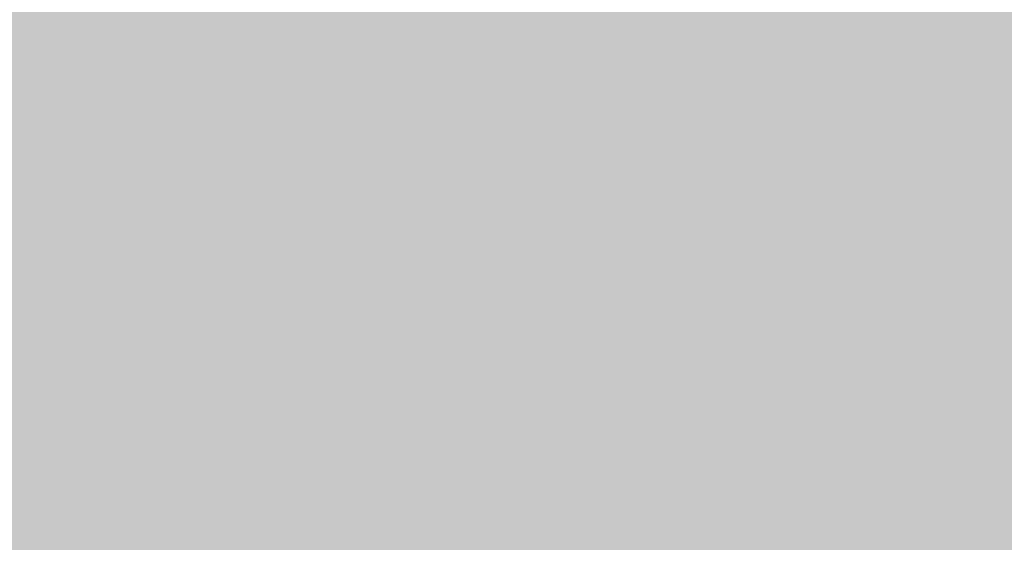
# Model space of a CAD drawing. Units: millimetres. Extents: x -22994 to 29398, y -19990 to 20176.
# Tile 104 of 135: x 223.11 to 237.22, y 87.07 to 94.56. Entities that reach past the tile are written whole.
import ezdxf
from ezdxf import colors
from ezdxf.entities.mleader import LeaderData, LeaderLine
from ezdxf.math import Vec2, Vec3

# ---------------------------------------------------------------- set-up
doc = ezdxf.new("R2010")
doc.units = ezdxf.units.MM
doc.header["$MEASUREMENT"] = 0
doc.layers.add('M-ANNO-TEXT', color=7, linetype='Continuous', lineweight=25)
doc.layers.add('M-DIMS', color=2, linetype='Continuous', lineweight=18)
doc.styles.get("Standard").update_dxf_attribs({"font": 'arial.ttf'})
doc.dimstyles.get("Standard").update_dxf_attribs({"dimtxt": 0.18, "dimasz": 10000, "dimexe": 0.18, "dimexo": 0.0625, "dimgap": 0.09, "dimtad": 0, "dimtih": 1, "dimtoh": 1, "dimdec": 0, "dimzin": 0, "dimdsep": 46, "dimtxsty": 'Standard', "dimcen": 0.09, "dimadec": 0, "dimazin": 0, "dimtfac": 1, "dimtdec": 0, "dimtofl": 0, "dimtmove": 0, "dimatfit": 3, "dimfxl": 1, "dimtolj": 1, "dimtzin": 0, "dimlwd": 30, "dimarcsym": 0})

# ---------------------------------------------------------------- blocks, each defined once
blk = doc.blocks.new('*D2')
at = {"layer": 'Defpoints', "color": 0, "transparency": 16777216}
for p in [(6.677, 10.271), (290.852, 10.271), (290.852, -5.079)]:
    blk.add_point(p, dxfattribs=at)
at = {"layer": 'M-DIMS', "color": 0, "lineweight": -2, "transparency": 16777216}
for p, q in [((6.677, 10.209), (6.677, -5.259)), ((290.852, 10.209), (290.852, -5.259))]:
    blk.add_line(p, q, dxfattribs=at)
at = {"layer": 'M-DIMS', "color": 0, "lineweight": 30, "transparency": 16777216}
for p, q in [((-9993.323, -5.079), (-19993.323, -5.079)), ((10290.852, -5.079), (20290.852, -5.079))]:
    blk.add_line(p, q, dxfattribs=at)
at = {"layer": 'M-DIMS', "color": 0, "transparency": 16777216}
for points in [[(-9993.323, 1661.588), (-9993.323, -1671.745), (6.677, -5.079)], [(10290.852, 1661.588), (10290.852, -1671.745), (290.852, -5.079)]]:
    blk.add_solid(points, dxfattribs=at)
at = {"layer": 'M-DIMS', "color": 0, "transparency": 16777216, "insert": (148.765, -5.079), "char_height": 0.18, "attachment_point": 5}
blk.add_mtext('\\A1;284.2', dxfattribs=at)
blk = doc.blocks.new('*D3')
at = {"layer": 'Defpoints', "color": 0, "transparency": 16777216}
for p in [(110.265, 204.165), (110.265, 176.366), (95.833, 127.967)]:
    blk.add_point(p, dxfattribs=at)
at = {"layer": 'M-DIMS', "color": 0, "lineweight": -2, "transparency": 16777216}
for p, q in [((95.833, 128.03), (95.833, 204.345)), ((110.265, 176.429), (110.265, 204.345))]:
    blk.add_line(p, q, dxfattribs=at)
at = {"layer": 'M-DIMS', "color": 0, "lineweight": 30, "transparency": 16777216}
for p, q in [((-9904.167, 204.165), (-19904.167, 204.165)), ((10110.265, 204.165), (20110.265, 204.165))]:
    blk.add_line(p, q, dxfattribs=at)
at = {"layer": 'M-DIMS', "color": 0, "transparency": 16777216}
for points in [[(-9904.167, 1870.832), (-9904.167, -1462.501), (95.833, 204.165)], [(10110.265, 1870.832), (10110.265, -1462.501), (110.265, 204.165)]]:
    blk.add_solid(points, dxfattribs=at)
at = {"layer": 'M-DIMS', "color": 0, "transparency": 16777216, "insert": (103.049, 204.165), "char_height": 0.18, "attachment_point": 5}
blk.add_mtext('\\A1;14.432', dxfattribs=at)
blk = doc.blocks.new('*D4')
at = {"layer": 'Defpoints', "color": 0, "transparency": 16777216}
for p in [(116.265, 204.165), (110.265, 176.366), (116.265, 176.366)]:
    blk.add_point(p, dxfattribs=at)
at = {"layer": 'M-DIMS', "color": 0, "lineweight": -2, "transparency": 16777216}
for p, q in [((110.265, 176.429), (110.265, 204.345)), ((116.265, 176.429), (116.265, 204.345))]:
    blk.add_line(p, q, dxfattribs=at)
at = {"layer": 'M-DIMS', "color": 0, "lineweight": 30, "transparency": 16777216}
for p, q in [((-9889.735, 204.165), (-19889.735, 204.165)), ((10116.265, 204.165), (20116.265, 204.165))]:
    blk.add_line(p, q, dxfattribs=at)
at = {"layer": 'M-DIMS', "color": 0, "transparency": 16777216}
for points in [[(-9889.735, 1870.832), (-9889.735, -1462.501), (110.265, 204.165)], [(10116.265, 1870.832), (10116.265, -1462.501), (116.265, 204.165)]]:
    blk.add_solid(points, dxfattribs=at)
at = {"layer": 'M-DIMS', "color": 0, "transparency": 16777216, "insert": (113.265, 204.165), "char_height": 0.18, "attachment_point": 5}
blk.add_mtext('\\A1;6', dxfattribs=at)
blk = doc.blocks.new('*D5')
at = {"layer": 'Defpoints', "color": 0, "transparency": 16777216}
for p in [(181.265, 204.165), (116.265, 176.366), (181.265, 176.366)]:
    blk.add_point(p, dxfattribs=at)
at = {"layer": 'M-DIMS', "color": 0, "lineweight": -2, "transparency": 16777216}
for p, q in [((116.265, 176.429), (116.265, 204.345)), ((181.265, 176.429), (181.265, 204.345))]:
    blk.add_line(p, q, dxfattribs=at)
at = {"layer": 'M-DIMS', "color": 0, "lineweight": 30, "transparency": 16777216}
for p, q in [((-9883.735, 204.165), (-19883.735, 204.165)), ((10181.265, 204.165), (20181.265, 204.165))]:
    blk.add_line(p, q, dxfattribs=at)
at = {"layer": 'M-DIMS', "color": 0, "transparency": 16777216}
for points in [[(-9883.735, 1870.832), (-9883.735, -1462.501), (116.265, 204.165)], [(10181.265, 1870.832), (10181.265, -1462.501), (181.265, 204.165)]]:
    blk.add_solid(points, dxfattribs=at)
at = {"layer": 'M-DIMS', "color": 0, "transparency": 16777216, "insert": (148.765, 204.165), "char_height": 0.18, "attachment_point": 5}
blk.add_mtext('\\A1;65', dxfattribs=at)
blk = doc.blocks.new('*D6')
at = {"layer": 'Defpoints', "color": 0, "transparency": 16777216}
for p in [(187.265, 204.165), (181.265, 176.366), (187.265, 176.366)]:
    blk.add_point(p, dxfattribs=at)
at = {"layer": 'M-DIMS', "color": 0, "lineweight": -2, "transparency": 16777216}
for p, q in [((181.265, 176.429), (181.265, 204.345)), ((187.265, 176.429), (187.265, 204.345))]:
    blk.add_line(p, q, dxfattribs=at)
at = {"layer": 'M-DIMS', "color": 0, "lineweight": 30, "transparency": 16777216}
for p, q in [((-9818.735, 204.165), (-19818.735, 204.165)), ((10187.265, 204.165), (20187.265, 204.165))]:
    blk.add_line(p, q, dxfattribs=at)
at = {"layer": 'M-DIMS', "color": 0, "transparency": 16777216}
for points in [[(-9818.735, 1870.832), (-9818.735, -1462.501), (181.265, 204.165)], [(10187.265, 1870.832), (10187.265, -1462.501), (187.265, 204.165)]]:
    blk.add_solid(points, dxfattribs=at)
at = {"layer": 'M-DIMS', "color": 0, "transparency": 16777216, "insert": (184.265, 204.165), "char_height": 0.18, "attachment_point": 5}
blk.add_mtext('\\A1;6', dxfattribs=at)
blk = doc.blocks.new('*D7')
at = {"layer": 'Defpoints', "color": 0, "transparency": 16777216}
for p in [(201.697, 204.165), (187.265, 176.366), (201.697, 127.967)]:
    blk.add_point(p, dxfattribs=at)
at = {"layer": 'M-DIMS', "color": 0, "lineweight": -2, "transparency": 16777216}
for p, q in [((187.265, 176.429), (187.265, 204.345)), ((201.697, 128.03), (201.697, 204.345))]:
    blk.add_line(p, q, dxfattribs=at)
at = {"layer": 'M-DIMS', "color": 0, "lineweight": 30, "transparency": 16777216}
for p, q in [((-9812.735, 204.165), (-19812.735, 204.165)), ((10201.697, 204.165), (20201.697, 204.165))]:
    blk.add_line(p, q, dxfattribs=at)
at = {"layer": 'M-DIMS', "color": 0, "transparency": 16777216}
for points in [[(-9812.735, 1870.832), (-9812.735, -1462.501), (187.265, 204.165)], [(10201.697, 1870.832), (10201.697, -1462.501), (201.697, 204.165)]]:
    blk.add_solid(points, dxfattribs=at)
at = {"layer": 'M-DIMS', "color": 0, "transparency": 16777216, "insert": (194.481, 204.165), "char_height": 0.18, "attachment_point": 5}
blk.add_mtext('\\A1;14.432', dxfattribs=at)
blk = doc.blocks.new('*D8')
at = {"layer": 'Defpoints', "color": 0, "transparency": 16777216}
for p in [(227.648, 204.165), (227.648, 146.73), (201.697, 127.967)]:
    blk.add_point(p, dxfattribs=at)
at = {"layer": 'M-DIMS', "color": 0, "lineweight": -2, "transparency": 16777216}
for p, q in [((201.697, 128.03), (201.697, 204.345)), ((227.648, 146.792), (227.648, 204.345))]:
    blk.add_line(p, q, dxfattribs=at)
at = {"layer": 'M-DIMS', "color": 0, "lineweight": 30, "transparency": 16777216}
for p, q in [((-9798.303, 204.165), (-19798.303, 204.165)), ((10227.648, 204.165), (20227.648, 204.165))]:
    blk.add_line(p, q, dxfattribs=at)
at = {"layer": 'M-DIMS', "color": 0, "transparency": 16777216}
for points in [[(-9798.303, 1870.832), (-9798.303, -1462.501), (201.697, 204.165)], [(10227.648, 1870.832), (10227.648, -1462.501), (227.648, 204.165)]]:
    blk.add_solid(points, dxfattribs=at)
at = {"layer": 'M-DIMS', "color": 0, "transparency": 16777216, "insert": (214.673, 204.165), "char_height": 0.18, "attachment_point": 5}
blk.add_mtext('\\A1;25.95', dxfattribs=at)
blk = doc.blocks.new('*D9')
at = {"layer": 'Defpoints', "color": 0, "transparency": 16777216}
for p in [(187.265, 176.366), (306.202, 176.366), (290.852, 10.271)]:
    blk.add_point(p, dxfattribs=at)
at = {"layer": 'M-DIMS', "color": 0, "lineweight": 30, "transparency": 16777216}
for p, q in [((306.202, 10176.366), (306.202, 20176.366)), ((306.202, -9989.729), (306.202, -19989.729))]:
    blk.add_line(p, q, dxfattribs=at)
at = {"layer": 'M-DIMS', "color": 0, "lineweight": -2, "transparency": 16777216}
for p, q in [((187.327, 176.366), (306.382, 176.366)), ((290.915, 10.271), (306.382, 10.271))]:
    blk.add_line(p, q, dxfattribs=at)
at = {"layer": 'M-DIMS', "color": 0, "transparency": 16777216}
for points in [[(-1360.465, 10176.366), (1972.869, 10176.366), (306.202, 176.366)], [(-1360.465, -9989.729), (1972.869, -9989.729), (306.202, 10.271)]]:
    blk.add_solid(points, dxfattribs=at)
at = {"layer": 'M-DIMS', "color": 0, "transparency": 16777216, "insert": (306.202, 93.319), "char_height": 0.18, "attachment_point": 5}
blk.add_mtext('\\A1;166.1', dxfattribs=at)
blk = doc.blocks.new('*D10')
at = {"layer": 'Defpoints', "color": 0, "transparency": 16777216}
for p in [(125.65, 136.071), (133.346, 136.071), (133.346, -5.079)]:
    blk.add_point(p, dxfattribs=at)
at = {"layer": 'M-DIMS', "color": 0, "lineweight": -2, "transparency": 16777216}
for p, q in [((125.65, 136.009), (125.65, -5.259)), ((133.346, 136.009), (133.346, -5.259))]:
    blk.add_line(p, q, dxfattribs=at)
at = {"layer": 'M-DIMS', "color": 0, "lineweight": 30, "transparency": 16777216}
for p, q in [((-9874.35, -5.079), (-19874.35, -5.079)), ((10133.346, -5.079), (20133.346, -5.079))]:
    blk.add_line(p, q, dxfattribs=at)
at = {"layer": 'M-DIMS', "color": 0, "transparency": 16777216}
for points in [[(-9874.35, 1661.588), (-9874.35, -1671.745), (125.65, -5.079)], [(10133.346, 1661.588), (10133.346, -1671.745), (133.346, -5.079)]]:
    blk.add_solid(points, dxfattribs=at)
at = {"layer": 'M-DIMS', "color": 0, "transparency": 16777216, "insert": (129.498, -5.079), "char_height": 0.18, "attachment_point": 5}
blk.add_mtext('\\A1;7.696', dxfattribs=at)
blk = doc.blocks.new('*D11')
at = {"layer": 'Defpoints', "color": 0, "transparency": 16777216}
for p in [(133.346, 136.071), (135.65, 136.071), (135.65, -5.079)]:
    blk.add_point(p, dxfattribs=at)
at = {"layer": 'M-DIMS', "color": 0, "lineweight": -2, "transparency": 16777216}
for p, q in [((133.346, 136.009), (133.346, -5.259)), ((135.65, 136.009), (135.65, -5.259))]:
    blk.add_line(p, q, dxfattribs=at)
at = {"layer": 'M-DIMS', "color": 0, "lineweight": 30, "transparency": 16777216}
for p, q in [((-9866.654, -5.079), (-19866.654, -5.079)), ((10135.65, -5.079), (20135.65, -5.079))]:
    blk.add_line(p, q, dxfattribs=at)
at = {"layer": 'M-DIMS', "color": 0, "transparency": 16777216}
for points in [[(-9866.654, 1661.588), (-9866.654, -1671.745), (133.346, -5.079)], [(10135.65, 1661.588), (10135.65, -1671.745), (135.65, -5.079)]]:
    blk.add_solid(points, dxfattribs=at)
at = {"layer": 'M-DIMS', "color": 0, "transparency": 16777216, "insert": (134.498, -5.079), "char_height": 0.18, "attachment_point": 5}
blk.add_mtext('\\A1;2.304', dxfattribs=at)
blk = doc.blocks.new('*D12')
at = {"layer": 'Defpoints', "color": 0, "transparency": 16777216}
for p in [(135.65, 136.071), (145.65, 136.071), (145.65, -5.079)]:
    blk.add_point(p, dxfattribs=at)
at = {"layer": 'M-DIMS', "color": 0, "lineweight": -2, "transparency": 16777216}
for p, q in [((135.65, 136.009), (135.65, -5.259)), ((145.65, 136.009), (145.65, -5.259))]:
    blk.add_line(p, q, dxfattribs=at)
at = {"layer": 'M-DIMS', "color": 0, "lineweight": 30, "transparency": 16777216}
for p, q in [((-9864.35, -5.079), (-19864.35, -5.079)), ((10145.65, -5.079), (20145.65, -5.079))]:
    blk.add_line(p, q, dxfattribs=at)
at = {"layer": 'M-DIMS', "color": 0, "transparency": 16777216}
for points in [[(-9864.35, 1661.588), (-9864.35, -1671.745), (135.65, -5.079)], [(10145.65, 1661.588), (10145.65, -1671.745), (145.65, -5.079)]]:
    blk.add_solid(points, dxfattribs=at)
at = {"layer": 'M-DIMS', "color": 0, "transparency": 16777216, "insert": (140.65, -5.079), "char_height": 0.18, "attachment_point": 5}
blk.add_mtext('\\A1;10', dxfattribs=at)
blk = doc.blocks.new('*D13')
at = {"layer": 'Defpoints', "color": 0, "transparency": 16777216}
for p in [(145.65, 136.071), (155.65, 136.071), (155.65, -5.079)]:
    blk.add_point(p, dxfattribs=at)
at = {"layer": 'M-DIMS', "color": 0, "lineweight": -2, "transparency": 16777216}
for p, q in [((145.65, 136.009), (145.65, -5.259)), ((155.65, 136.009), (155.65, -5.259))]:
    blk.add_line(p, q, dxfattribs=at)
at = {"layer": 'M-DIMS', "color": 0, "lineweight": 30, "transparency": 16777216}
for p, q in [((-9854.35, -5.079), (-19854.35, -5.079)), ((10155.65, -5.079), (20155.65, -5.079))]:
    blk.add_line(p, q, dxfattribs=at)
at = {"layer": 'M-DIMS', "color": 0, "transparency": 16777216}
for points in [[(-9854.35, 1661.588), (-9854.35, -1671.745), (145.65, -5.079)], [(10155.65, 1661.588), (10155.65, -1671.745), (155.65, -5.079)]]:
    blk.add_solid(points, dxfattribs=at)
at = {"layer": 'M-DIMS', "color": 0, "transparency": 16777216, "insert": (150.65, -5.079), "char_height": 0.18, "attachment_point": 5}
blk.add_mtext('\\A1;10', dxfattribs=at)
blk = doc.blocks.new('*D14')
at = {"layer": 'Defpoints', "color": 0, "transparency": 16777216}
for p in [(155.65, 136.071), (165.65, 136.071), (165.65, -5.079)]:
    blk.add_point(p, dxfattribs=at)
at = {"layer": 'M-DIMS', "color": 0, "lineweight": -2, "transparency": 16777216}
for p, q in [((155.65, 136.009), (155.65, -5.259)), ((165.65, 136.009), (165.65, -5.259))]:
    blk.add_line(p, q, dxfattribs=at)
at = {"layer": 'M-DIMS', "color": 0, "lineweight": 30, "transparency": 16777216}
for p, q in [((-9844.35, -5.079), (-19844.35, -5.079)), ((10165.65, -5.079), (20165.65, -5.079))]:
    blk.add_line(p, q, dxfattribs=at)
at = {"layer": 'M-DIMS', "color": 0, "transparency": 16777216}
for points in [[(-9844.35, 1661.588), (-9844.35, -1671.745), (155.65, -5.079)], [(10165.65, 1661.588), (10165.65, -1671.745), (165.65, -5.079)]]:
    blk.add_solid(points, dxfattribs=at)
at = {"layer": 'M-DIMS', "color": 0, "transparency": 16777216, "insert": (160.65, -5.079), "char_height": 0.18, "attachment_point": 5}
blk.add_mtext('\\A1;10', dxfattribs=at)
blk = doc.blocks.new('*D15')
at = {"layer": 'Defpoints', "color": 0, "transparency": 16777216}
for p in [(173.346, 154.788), (173.346, 136.071), (306.202, 136.071)]:
    blk.add_point(p, dxfattribs=at)
at = {"layer": 'M-DIMS', "color": 0, "lineweight": 30, "transparency": 16777216}
for p, q in [((306.202, 10154.788), (306.202, 20154.788)), ((306.202, -9863.929), (306.202, -19863.929))]:
    blk.add_line(p, q, dxfattribs=at)
at = {"layer": 'M-DIMS', "color": 0, "lineweight": -2, "transparency": 16777216}
for p, q in [((173.408, 154.788), (306.382, 154.788)), ((173.408, 136.071), (306.382, 136.071))]:
    blk.add_line(p, q, dxfattribs=at)
at = {"layer": 'M-DIMS', "color": 0, "transparency": 16777216}
for points in [[(-1360.465, 10154.788), (1972.869, 10154.788), (306.202, 154.788)], [(-1360.465, -9863.929), (1972.869, -9863.929), (306.202, 136.071)]]:
    blk.add_solid(points, dxfattribs=at)
at = {"layer": 'M-DIMS', "color": 0, "transparency": 16777216, "insert": (306.202, 145.43), "char_height": 0.18, "attachment_point": 5}
blk.add_mtext('\\A1;18.717', dxfattribs=at)
blk = doc.blocks.new('*D16')
at = {"layer": 'Defpoints', "color": 0, "transparency": 16777216}
for p in [(120.17, 204.165), (110.466, 48.035), (120.17, 48.035)]:
    blk.add_point(p, dxfattribs=at)
at = {"layer": 'M-DIMS', "color": 0, "lineweight": -2, "transparency": 16777216}
for p, q in [((110.466, 48.097), (110.466, 204.345)), ((120.17, 48.097), (120.17, 204.345))]:
    blk.add_line(p, q, dxfattribs=at)
at = {"layer": 'M-DIMS', "color": 0, "lineweight": 30, "transparency": 16777216}
for p, q in [((-9889.534, 204.165), (-19889.534, 204.165)), ((10120.17, 204.165), (20120.17, 204.165))]:
    blk.add_line(p, q, dxfattribs=at)
at = {"layer": 'M-DIMS', "color": 0, "transparency": 16777216}
for points in [[(-9889.534, 1870.832), (-9889.534, -1462.501), (110.466, 204.165)], [(10120.17, 1870.832), (10120.17, -1462.501), (120.17, 204.165)]]:
    blk.add_solid(points, dxfattribs=at)
at = {"layer": 'M-DIMS', "color": 0, "transparency": 16777216, "insert": (115.318, 204.165), "char_height": 0.18, "attachment_point": 5}
blk.add_mtext('\\A1;9.704', dxfattribs=at)
blk = doc.blocks.new('*D17')
at = {"layer": 'Defpoints', "color": 0, "transparency": 16777216}
for p in [(126.17, 204.165), (120.17, 48.035), (126.17, 48.035)]:
    blk.add_point(p, dxfattribs=at)
at = {"layer": 'M-DIMS', "color": 0, "lineweight": -2, "transparency": 16777216}
for p, q in [((120.17, 48.097), (120.17, 204.345)), ((126.17, 48.097), (126.17, 204.345))]:
    blk.add_line(p, q, dxfattribs=at)
at = {"layer": 'M-DIMS', "color": 0, "lineweight": 30, "transparency": 16777216}
for p, q in [((-9879.83, 204.165), (-19879.83, 204.165)), ((10126.17, 204.165), (20126.17, 204.165))]:
    blk.add_line(p, q, dxfattribs=at)
at = {"layer": 'M-DIMS', "color": 0, "transparency": 16777216}
for points in [[(-9879.83, 1870.832), (-9879.83, -1462.501), (120.17, 204.165)], [(10126.17, 1870.832), (10126.17, -1462.501), (126.17, 204.165)]]:
    blk.add_solid(points, dxfattribs=at)
at = {"layer": 'M-DIMS', "color": 0, "transparency": 16777216, "insert": (123.17, 204.165), "char_height": 0.18, "attachment_point": 5}
blk.add_mtext('\\A1;6', dxfattribs=at)
blk = doc.blocks.new('*D18')
at = {"layer": 'Defpoints', "color": 0, "transparency": 16777216}
for p in [(132.17, 204.165), (126.17, 48.035), (132.17, 48.035)]:
    blk.add_point(p, dxfattribs=at)
at = {"layer": 'M-DIMS', "color": 0, "lineweight": -2, "transparency": 16777216}
for p, q in [((126.17, 48.097), (126.17, 204.345)), ((132.17, 48.097), (132.17, 204.345))]:
    blk.add_line(p, q, dxfattribs=at)
at = {"layer": 'M-DIMS', "color": 0, "lineweight": 30, "transparency": 16777216}
for p, q in [((-9873.83, 204.165), (-19873.83, 204.165)), ((10132.17, 204.165), (20132.17, 204.165))]:
    blk.add_line(p, q, dxfattribs=at)
at = {"layer": 'M-DIMS', "color": 0, "transparency": 16777216}
for points in [[(-9873.83, 1870.832), (-9873.83, -1462.501), (126.17, 204.165)], [(10132.17, 1870.832), (10132.17, -1462.501), (132.17, 204.165)]]:
    blk.add_solid(points, dxfattribs=at)
at = {"layer": 'M-DIMS', "color": 0, "transparency": 16777216, "insert": (129.17, 204.165), "char_height": 0.18, "attachment_point": 5}
blk.add_mtext('\\A1;6', dxfattribs=at)
blk = doc.blocks.new('*D19')
at = {"layer": 'Defpoints', "color": 0, "transparency": 16777216}
for p in [(138.17, 204.165), (132.17, 48.035), (138.17, 48.035)]:
    blk.add_point(p, dxfattribs=at)
at = {"layer": 'M-DIMS', "color": 0, "lineweight": -2, "transparency": 16777216}
for p, q in [((132.17, 48.097), (132.17, 204.345)), ((138.17, 48.097), (138.17, 204.345))]:
    blk.add_line(p, q, dxfattribs=at)
at = {"layer": 'M-DIMS', "color": 0, "lineweight": 30, "transparency": 16777216}
for p, q in [((-9867.83, 204.165), (-19867.83, 204.165)), ((10138.17, 204.165), (20138.17, 204.165))]:
    blk.add_line(p, q, dxfattribs=at)
at = {"layer": 'M-DIMS', "color": 0, "transparency": 16777216}
for points in [[(-9867.83, 1870.832), (-9867.83, -1462.501), (132.17, 204.165)], [(10138.17, 1870.832), (10138.17, -1462.501), (138.17, 204.165)]]:
    blk.add_solid(points, dxfattribs=at)
at = {"layer": 'M-DIMS', "color": 0, "transparency": 16777216, "insert": (135.17, 204.165), "char_height": 0.18, "attachment_point": 5}
blk.add_mtext('\\A1;6', dxfattribs=at)
blk = doc.blocks.new('*D20')
at = {"layer": 'Defpoints', "color": 0, "transparency": 16777216}
for p in [(144.17, 204.165), (138.17, 48.035), (144.17, 48.035)]:
    blk.add_point(p, dxfattribs=at)
at = {"layer": 'M-DIMS', "color": 0, "lineweight": -2, "transparency": 16777216}
for p, q in [((138.17, 48.097), (138.17, 204.345)), ((144.17, 48.097), (144.17, 204.345))]:
    blk.add_line(p, q, dxfattribs=at)
at = {"layer": 'M-DIMS', "color": 0, "lineweight": 30, "transparency": 16777216}
for p, q in [((-9861.83, 204.165), (-19861.83, 204.165)), ((10144.17, 204.165), (20144.17, 204.165))]:
    blk.add_line(p, q, dxfattribs=at)
at = {"layer": 'M-DIMS', "color": 0, "transparency": 16777216}
for points in [[(-9861.83, 1870.832), (-9861.83, -1462.501), (138.17, 204.165)], [(10144.17, 1870.832), (10144.17, -1462.501), (144.17, 204.165)]]:
    blk.add_solid(points, dxfattribs=at)
at = {"layer": 'M-DIMS', "color": 0, "transparency": 16777216, "insert": (141.17, 204.165), "char_height": 0.18, "attachment_point": 5}
blk.add_mtext('\\A1;6', dxfattribs=at)
blk = doc.blocks.new('*D21')
at = {"layer": 'Defpoints', "color": 0, "transparency": 16777216}
for p in [(149.116, 204.165), (144.17, 48.035), (149.116, 48.035)]:
    blk.add_point(p, dxfattribs=at)
at = {"layer": 'M-DIMS', "color": 0, "lineweight": -2, "transparency": 16777216}
for p, q in [((144.17, 48.097), (144.17, 204.345)), ((149.116, 48.097), (149.116, 204.345))]:
    blk.add_line(p, q, dxfattribs=at)
at = {"layer": 'M-DIMS', "color": 0, "lineweight": 30, "transparency": 16777216}
for p, q in [((-9855.83, 204.165), (-19855.83, 204.165)), ((10149.116, 204.165), (20149.116, 204.165))]:
    blk.add_line(p, q, dxfattribs=at)
at = {"layer": 'M-DIMS', "color": 0, "transparency": 16777216}
for points in [[(-9855.83, 1870.832), (-9855.83, -1462.501), (144.17, 204.165)], [(10149.116, 1870.832), (10149.116, -1462.501), (149.116, 204.165)]]:
    blk.add_solid(points, dxfattribs=at)
at = {"layer": 'M-DIMS', "color": 0, "transparency": 16777216, "insert": (146.643, 204.165), "char_height": 0.18, "attachment_point": 5}
blk.add_mtext('\\A1;4.945', dxfattribs=at)
blk = doc.blocks.new('*D22')
at = {"layer": 'Defpoints', "color": 0, "transparency": 16777216}
for p in [(149.116, 30.99), (155.116, 30.99), (155.116, -5.079)]:
    blk.add_point(p, dxfattribs=at)
at = {"layer": 'M-DIMS', "color": 0, "lineweight": -2, "transparency": 16777216}
for p, q in [((149.116, 30.927), (149.116, -5.259)), ((155.116, 30.927), (155.116, -5.259))]:
    blk.add_line(p, q, dxfattribs=at)
at = {"layer": 'M-DIMS', "color": 0, "lineweight": 30, "transparency": 16777216}
for p, q in [((-9850.884, -5.079), (-19850.884, -5.079)), ((10155.116, -5.079), (20155.116, -5.079))]:
    blk.add_line(p, q, dxfattribs=at)
at = {"layer": 'M-DIMS', "color": 0, "transparency": 16777216}
for points in [[(-9850.884, 1661.588), (-9850.884, -1671.745), (149.116, -5.079)], [(10155.116, 1661.588), (10155.116, -1671.745), (155.116, -5.079)]]:
    blk.add_solid(points, dxfattribs=at)
at = {"layer": 'M-DIMS', "color": 0, "transparency": 16777216, "insert": (152.116, -5.079), "char_height": 0.18, "attachment_point": 5}
blk.add_mtext('\\A1;6', dxfattribs=at)
blk = doc.blocks.new('*D23')
at = {"layer": 'Defpoints', "color": 0, "transparency": 16777216}
for p in [(155.116, 30.99), (161.116, 30.99), (161.116, -5.079)]:
    blk.add_point(p, dxfattribs=at)
at = {"layer": 'M-DIMS', "color": 0, "lineweight": -2, "transparency": 16777216}
for p, q in [((155.116, 30.927), (155.116, -5.259)), ((161.116, 30.927), (161.116, -5.259))]:
    blk.add_line(p, q, dxfattribs=at)
at = {"layer": 'M-DIMS', "color": 0, "lineweight": 30, "transparency": 16777216}
for p, q in [((-9844.884, -5.079), (-19844.884, -5.079)), ((10161.116, -5.079), (20161.116, -5.079))]:
    blk.add_line(p, q, dxfattribs=at)
at = {"layer": 'M-DIMS', "color": 0, "transparency": 16777216}
for points in [[(-9844.884, 1661.588), (-9844.884, -1671.745), (155.116, -5.079)], [(10161.116, 1661.588), (10161.116, -1671.745), (161.116, -5.079)]]:
    blk.add_solid(points, dxfattribs=at)
at = {"layer": 'M-DIMS', "color": 0, "transparency": 16777216, "insert": (158.116, -5.079), "char_height": 0.18, "attachment_point": 5}
blk.add_mtext('\\A1;6', dxfattribs=at)
blk = doc.blocks.new('*D24')
at = {"layer": 'Defpoints', "color": 0, "transparency": 16777216}
for p in [(161.116, 30.99), (166.439, 30.99), (166.439, -5.079)]:
    blk.add_point(p, dxfattribs=at)
at = {"layer": 'M-DIMS', "color": 0, "lineweight": -2, "transparency": 16777216}
for p, q in [((161.116, 30.927), (161.116, -5.259)), ((166.439, 30.927), (166.439, -5.259))]:
    blk.add_line(p, q, dxfattribs=at)
at = {"layer": 'M-DIMS', "color": 0, "lineweight": 30, "transparency": 16777216}
for p, q in [((-9838.884, -5.079), (-19838.884, -5.079)), ((10166.439, -5.079), (20166.439, -5.079))]:
    blk.add_line(p, q, dxfattribs=at)
at = {"layer": 'M-DIMS', "color": 0, "transparency": 16777216}
for points in [[(-9838.884, 1661.588), (-9838.884, -1671.745), (161.116, -5.079)], [(10166.439, 1661.588), (10166.439, -1671.745), (166.439, -5.079)]]:
    blk.add_solid(points, dxfattribs=at)
at = {"layer": 'M-DIMS', "color": 0, "transparency": 16777216, "insert": (163.777, -5.079), "char_height": 0.18, "attachment_point": 5}
blk.add_mtext('\\A1;5.323', dxfattribs=at)
blk = doc.blocks.new('*D25')
at = {"layer": 'Defpoints', "color": 0, "transparency": 16777216}
for p in [(166.439, 30.99), (172.439, 30.99), (172.439, -5.079)]:
    blk.add_point(p, dxfattribs=at)
at = {"layer": 'M-DIMS', "color": 0, "lineweight": -2, "transparency": 16777216}
for p, q in [((166.439, 30.927), (166.439, -5.259)), ((172.439, 30.927), (172.439, -5.259))]:
    blk.add_line(p, q, dxfattribs=at)
at = {"layer": 'M-DIMS', "color": 0, "lineweight": 30, "transparency": 16777216}
for p, q in [((-9833.561, -5.079), (-19833.561, -5.079)), ((10172.439, -5.079), (20172.439, -5.079))]:
    blk.add_line(p, q, dxfattribs=at)
at = {"layer": 'M-DIMS', "color": 0, "transparency": 16777216}
for points in [[(-9833.561, 1661.588), (-9833.561, -1671.745), (166.439, -5.079)], [(10172.439, 1661.588), (10172.439, -1671.745), (172.439, -5.079)]]:
    blk.add_solid(points, dxfattribs=at)
at = {"layer": 'M-DIMS', "color": 0, "transparency": 16777216, "insert": (169.439, -5.079), "char_height": 0.18, "attachment_point": 5}
blk.add_mtext('\\A1;6', dxfattribs=at)
blk = doc.blocks.new('*D26')
at = {"layer": 'Defpoints', "color": 0, "transparency": 16777216}
for p in [(172.439, 30.99), (178.439, 30.99), (178.439, -5.079)]:
    blk.add_point(p, dxfattribs=at)
at = {"layer": 'M-DIMS', "color": 0, "lineweight": -2, "transparency": 16777216}
for p, q in [((172.439, 30.927), (172.439, -5.259)), ((178.439, 30.927), (178.439, -5.259))]:
    blk.add_line(p, q, dxfattribs=at)
at = {"layer": 'M-DIMS', "color": 0, "lineweight": 30, "transparency": 16777216}
for p, q in [((-9827.561, -5.079), (-19827.561, -5.079)), ((10178.439, -5.079), (20178.439, -5.079))]:
    blk.add_line(p, q, dxfattribs=at)
at = {"layer": 'M-DIMS', "color": 0, "transparency": 16777216}
for points in [[(-9827.561, 1661.588), (-9827.561, -1671.745), (172.439, -5.079)], [(10178.439, 1661.588), (10178.439, -1671.745), (178.439, -5.079)]]:
    blk.add_solid(points, dxfattribs=at)
at = {"layer": 'M-DIMS', "color": 0, "transparency": 16777216, "insert": (175.439, -5.079), "char_height": 0.18, "attachment_point": 5}
blk.add_mtext('\\A1;6', dxfattribs=at)
blk = doc.blocks.new('*D27')
at = {"layer": 'Defpoints', "color": 0, "transparency": 16777216}
for p in [(178.439, 30.99), (188.117, 30.99), (188.117, -5.079)]:
    blk.add_point(p, dxfattribs=at)
at = {"layer": 'M-DIMS', "color": 0, "lineweight": -2, "transparency": 16777216}
for p, q in [((178.439, 30.927), (178.439, -5.259)), ((188.117, 30.927), (188.117, -5.259))]:
    blk.add_line(p, q, dxfattribs=at)
at = {"layer": 'M-DIMS', "color": 0, "lineweight": 30, "transparency": 16777216}
for p, q in [((-9821.561, -5.079), (-19821.561, -5.079)), ((10188.117, -5.079), (20188.117, -5.079))]:
    blk.add_line(p, q, dxfattribs=at)
at = {"layer": 'M-DIMS', "color": 0, "transparency": 16777216}
for points in [[(-9821.561, 1661.588), (-9821.561, -1671.745), (178.439, -5.079)], [(10188.117, 1661.588), (10188.117, -1671.745), (188.117, -5.079)]]:
    blk.add_solid(points, dxfattribs=at)
at = {"layer": 'M-DIMS', "color": 0, "transparency": 16777216, "insert": (183.278, -5.079), "char_height": 0.18, "attachment_point": 5}
blk.add_mtext('\\A1;9.679', dxfattribs=at)
blk = doc.blocks.new('*D28')
at = {"layer": 'Defpoints', "color": 0, "transparency": 16777216}
for p in [(188.117, 48.035), (306.202, 48.035), (188.117, 30.99)]:
    blk.add_point(p, dxfattribs=at)
at = {"layer": 'M-DIMS', "color": 0, "lineweight": 30, "transparency": 16777216}
for p, q in [((306.202, 10048.035), (306.202, 20048.035)), ((306.202, -9969.01), (306.202, -19969.01))]:
    blk.add_line(p, q, dxfattribs=at)
at = {"layer": 'M-DIMS', "color": 0, "lineweight": -2, "transparency": 16777216}
for p, q in [((188.18, 48.035), (306.382, 48.035)), ((188.18, 30.99), (306.382, 30.99))]:
    blk.add_line(p, q, dxfattribs=at)
at = {"layer": 'M-DIMS', "color": 0, "transparency": 16777216}
for points in [[(-1360.465, 10048.035), (1972.869, 10048.035), (306.202, 48.035)], [(-1360.465, -9969.01), (1972.869, -9969.01), (306.202, 30.99)]]:
    blk.add_solid(points, dxfattribs=at)
at = {"layer": 'M-DIMS', "color": 0, "transparency": 16777216, "insert": (306.202, 39.512), "char_height": 0.18, "attachment_point": 5}
blk.add_mtext('\\A1;17.045', dxfattribs=at)
blk = doc.blocks.new('*D29')
at = {"layer": 'Defpoints', "color": 0, "transparency": 16777216}
for p in [(36.801, 80.045), (64.03, 80.045)]:
    blk.add_point(p, dxfattribs=at)
at = {"layer": 'M-DIMS', "color": 0, "lineweight": -2, "transparency": 16777216}
for p, q in [((50.325, 80.045), (50.505, 80.045)), ((50.415, 79.955), (50.415, 80.135))]:
    blk.add_line(p, q, dxfattribs=at)
at = {"layer": 'M-DIMS', "color": 0, "lineweight": 30, "transparency": 16777216}
blk.add_line((20064.03, 80.03), (10064.03, 80.038), dxfattribs=at)
at = {"layer": 'M-DIMS', "color": 0, "transparency": 16777216}
blk.add_solid([(10064.031, 1746.704), (10064.028, -1586.629), (64.03, 80.045)], dxfattribs=at)
at = {"layer": 'M-DIMS', "color": 0, "transparency": 16777216, "insert": (20064.521, 80.03), "char_height": 0.18, "attachment_point": 5}
blk.add_mtext('\\A1;∅27.23', dxfattribs=at)
blk = doc.blocks.new('*D30')
at = {"layer": 'Defpoints', "color": 0, "transparency": 16777216}
for p in [(216.315, 146.729), (238.982, 146.73)]:
    blk.add_point(p, dxfattribs=at)
at = {"layer": 'M-DIMS', "color": 0, "lineweight": 30, "transparency": 16777216}
blk.add_line((20238.982, 147.496), (10238.982, 147.113), dxfattribs=at)
at = {"layer": 'M-DIMS', "color": 0, "lineweight": -2, "transparency": 16777216}
for p, q in [((227.648, 146.64), (227.648, 146.82)), ((227.558, 146.73), (227.738, 146.73))]:
    blk.add_line(p, q, dxfattribs=at)
at = {"layer": 'M-DIMS', "color": 0, "transparency": 16777216}
blk.add_solid([(10238.918, 1813.78), (10239.046, -1519.554), (238.982, 146.73)], dxfattribs=at)
at = {"layer": 'M-DIMS', "color": 0, "transparency": 16777216, "insert": (20239.544, 147.496), "char_height": 0.18, "attachment_point": 5}
blk.add_mtext('\\A1;∅22.667', dxfattribs=at)
blk = doc.blocks.new('*D31')
at = {"layer": 'Defpoints', "color": 0, "transparency": 16777216}
for p in [(223.164, 146.729), (232.133, 146.73)]:
    blk.add_point(p, dxfattribs=at)
at = {"layer": 'M-DIMS', "color": 0, "lineweight": 30, "transparency": 16777216}
blk.add_line((20232.133, 148.666), (10232.133, 147.698), dxfattribs=at)
at = {"layer": 'M-DIMS', "color": 0, "lineweight": -2, "transparency": 16777216}
for p, q in [((227.648, 146.64), (227.648, 146.82)), ((227.558, 146.73), (227.738, 146.73))]:
    blk.add_line(p, q, dxfattribs=at)
at = {"layer": 'M-DIMS', "color": 0, "transparency": 16777216}
blk.add_solid([(10231.971, 1814.364), (10232.294, -1518.969), (232.133, 146.73)], dxfattribs=at)
at = {"layer": 'M-DIMS', "color": 0, "transparency": 16777216, "insert": (20232.625, 148.666), "char_height": 0.18, "attachment_point": 5}
blk.add_mtext('\\A1;∅8.969', dxfattribs=at)
blk = doc.blocks.new('*D33')
at = {"layer": 'Defpoints', "color": 0, "transparency": 16777216}
for p in [(229.561, 154.377), (232.997, 153.351)]:
    blk.add_point(p, dxfattribs=at)
at = {"layer": 'M-DIMS', "color": 0, "lineweight": -2, "transparency": 16777216}
for p, q in [((229.471, 154.377), (229.651, 154.377)), ((229.561, 154.287), (229.561, 154.467))]:
    blk.add_line(p, q, dxfattribs=at)
at = {"layer": 'M-DIMS', "color": 0, "lineweight": 30, "transparency": 16777216}
for p, q in [((19396.339, -5570.838), (9814.668, -2708.743)), ((29396.339, -5570.838), (19396.339, -5570.838))]:
    blk.add_line(p, q, dxfattribs=at)
at = {"layer": 'M-DIMS', "color": 0, "transparency": 16777216}
blk.add_solid([(10291.684, -1111.798), (9337.652, -4305.689), (232.997, 153.351)], dxfattribs=at)
at = {"layer": 'M-DIMS', "color": 0, "transparency": 16777216, "insert": (29397.012, -5570.838), "char_height": 0.18, "attachment_point": 5}
blk.add_mtext('\\A1;6X R3.586', dxfattribs=at)
blk = doc.blocks.new('*D36')
at = {"layer": 'Defpoints', "color": 0, "transparency": 16777216}
for p in [(46.39, 31.303), (46.387, 26.593)]:
    blk.add_point(p, dxfattribs=at)
at = {"layer": 'M-DIMS', "color": 0, "lineweight": 30, "transparency": 16777216}
for p, q in [((57.15, 20031.301), (51.77, 10031.302)), ((10057.15, 20031.301), (57.15, 20031.301))]:
    blk.add_line(p, q, dxfattribs=at)
at = {"layer": 'M-DIMS', "color": 0, "lineweight": -2, "transparency": 16777216}
for p, q in [((46.299, 28.948), (46.479, 28.948)), ((46.389, 28.858), (46.389, 29.038))]:
    blk.add_line(p, q, dxfattribs=at)
at = {"layer": 'M-DIMS', "color": 0, "transparency": 16777216}
blk.add_solid([(-1614.896, 10032.199), (1718.436, 10030.405), (46.39, 31.303)], dxfattribs=at)
at = {"layer": 'M-DIMS', "color": 0, "transparency": 16777216, "insert": (10057.554, 20031.301), "char_height": 0.18, "attachment_point": 5}
blk.add_mtext('\\A1;∅4.71', dxfattribs=at)
blk = doc.blocks.new('*D37')
at = {"layer": 'Defpoints', "color": 0, "transparency": 16777216}
for p in [(54.834, 118.615), (59.494, 118.614)]:
    blk.add_point(p, dxfattribs=at)
at = {"layer": 'M-DIMS', "color": 0, "lineweight": -2, "transparency": 16777216}
for p, q in [((57.164, 118.524), (57.164, 118.704)), ((57.074, 118.614), (57.254, 118.614))]:
    blk.add_line(p, q, dxfattribs=at)
at = {"layer": 'M-DIMS', "color": 0, "lineweight": 30, "transparency": 16777216}
blk.add_line((20059.493, 116.253), (10059.494, 117.434), dxfattribs=at)
at = {"layer": 'M-DIMS', "color": 0, "transparency": 16777216}
blk.add_solid([(10059.69, 1784.1), (10059.297, -1549.233), (59.494, 118.614)], dxfattribs=at)
at = {"layer": 'M-DIMS', "color": 0, "transparency": 16777216, "insert": (20059.985, 116.253), "char_height": 0.18, "attachment_point": 5}
blk.add_mtext('\\A1;∅4.659', dxfattribs=at)

msp = doc.modelspace()

# ---------------------------------------------------------------- dimensions: what is measured, and where the dimension line sits
at = {"layer": 'M-DIMS'}
for base, p1, p2, override, picture, middle in [((306.202, 176.3662), (290.852, 10.2713), (187.2647, 176.3662), {"dimdec": 1, "dimlfac": 1, "dimrnd": 0, "dimzin": 0, "dimdsep": 46, "dimlunit": 2}, '*D9', (306.202, 93.3187)), ((306.202, 136.0713), (173.3459, 154.788), (173.3459, 136.0713), {"dimdec": 3, "dimlfac": 1, "dimrnd": 0, "dimzin": 0, "dimdsep": 46, "dimlunit": 2}, '*D15', (306.202, 145.4297)), ((306.202, 48.0349), (188.1175, 30.9895), (188.1175, 48.0349), {"dimdec": 3, "dimlfac": 1, "dimrnd": 0, "dimzin": 0, "dimdsep": 46, "dimlunit": 2}, '*D28', (306.202, 39.5122))]:
    dim = msp.add_linear_dim(base=base, p1=p1, p2=p2, angle=90, dimstyle='Standard', override=override, dxfattribs=at)
    dim.commit()
    dim.dimension.update_dxf_attribs({"geometry": picture, "text_midpoint": middle})
for p1, p2, override, picture, middle in [((46.3875, 26.5934), (46.39, 31.3035), {"dimdec": 2, "dimlfac": 1, "dimrnd": 0, "dimzin": 0, "dimdsep": 46, "dimlunit": 2}, '*D36', (10057.5542, 20031.3006)), ((223.1641, 146.7291), (232.1328, 146.73), {"dimdec": 3, "dimlfac": 1, "dimrnd": 0, "dimzin": 0, "dimdsep": 46, "dimlunit": 2}, '*D31', (20232.1327, 148.6656)), ((216.3148, 146.7291), (238.9821, 146.73), {"dimdec": 3, "dimlfac": 1, "dimrnd": 0, "dimzin": 0, "dimdsep": 46, "dimlunit": 2}, '*D30', (20238.9821, 147.4959))]:
    dim = msp.add_diameter_dim_2p(p1=p1, p2=p2, dimstyle='Standard', override=override, dxfattribs=at)
    dim.commit()
    dim.dimension.update_dxf_attribs({"geometry": picture, "text_midpoint": middle, "dimtype": 163})
for base, p1, p2, override, picture, middle in [((110.2647, 204.1654), (95.8327, 127.967), (110.2647, 176.3662), {"dimdec": 3, "dimlfac": 1, "dimrnd": 0, "dimzin": 0, "dimdsep": 46, "dimlunit": 2}, '*D3', (103.0487, 204.1654)), ((116.2647, 204.1654), (110.2647, 176.3662), (116.2647, 176.3662), {"dimdec": 0, "dimlfac": 1, "dimrnd": 0, "dimzin": 0, "dimdsep": 46, "dimlunit": 2}, '*D4', (113.2647, 204.1654)), ((120.1702, 204.1654), (110.4658, 48.0349), (120.1702, 48.0349), {"dimdec": 3, "dimlfac": 1, "dimrnd": 0, "dimzin": 0, "dimdsep": 46, "dimlunit": 2}, '*D16', (115.318, 204.1654)), ((181.2647, 204.1654), (116.2647, 176.3662), (181.2647, 176.3662), {"dimdec": 0, "dimlfac": 1, "dimrnd": 0, "dimzin": 0, "dimdsep": 46, "dimlunit": 2}, '*D5', (148.7647, 204.1654)), ((126.1702, 204.1654), (120.1702, 48.0349), (126.1702, 48.0349), {"dimdec": 0, "dimlfac": 1, "dimrnd": 0, "dimzin": 0, "dimdsep": 46, "dimlunit": 2}, '*D17', (123.1702, 204.1654)), ((132.1702, 204.1654), (126.1702, 48.0349), (132.1702, 48.0349), {"dimdec": 0, "dimlfac": 1, "dimrnd": 0, "dimzin": 0, "dimdsep": 46, "dimlunit": 2}, '*D18', (129.1702, 204.1654)), ((138.1702, 204.1654), (132.1702, 48.0349), (138.1702, 48.0349), {"dimdec": 0, "dimlfac": 1, "dimrnd": 0, "dimzin": 0, "dimdsep": 46, "dimlunit": 2}, '*D19', (135.1702, 204.1654)), ((144.1702, 204.1654), (138.1702, 48.0349), (144.1702, 48.0349), {"dimdec": 0, "dimlfac": 1, "dimrnd": 0, "dimzin": 0, "dimdsep": 46, "dimlunit": 2}, '*D20', (141.1702, 204.1654)), ((149.11567, 204.16539), (144.17023, 48.03494), (149.11567, 48.03494), {"dimdec": 3, "dimlfac": 1, "dimrnd": 0, "dimzin": 0, "dimdsep": 46, "dimlunit": 2}, '*D21', (146.64295, 204.16539)), ((187.2647, 204.1654), (181.2647, 176.3662), (187.2647, 176.3662), {"dimdec": 0, "dimlfac": 1, "dimrnd": 0, "dimzin": 0, "dimdsep": 46, "dimlunit": 2}, '*D6', (184.2647, 204.1654)), ((201.6967, 204.1654), (187.2647, 176.3662), (201.6967, 127.967), {"dimdec": 3, "dimlfac": 1, "dimrnd": 0, "dimzin": 0, "dimdsep": 46, "dimlunit": 2}, '*D7', (194.4807, 204.1654)), ((227.6485, 204.1654), (201.6967, 127.967), (227.6485, 146.7296), {"dimdec": 2, "dimlfac": 1, "dimrnd": 0, "dimzin": 0, "dimdsep": 46, "dimlunit": 2}, '*D8', (214.6726, 204.1654)), ((290.852, -5.0787), (6.6773, 10.2713), (290.852, 10.2713), {"dimdec": 1, "dimlfac": 1, "dimrnd": 0, "dimzin": 0, "dimdsep": 46, "dimlunit": 2}, '*D2', (148.7647, -5.0787)), ((133.3459, -5.0787), (125.6498, 136.0713), (133.3459, 136.0713), {"dimdec": 3, "dimlfac": 1, "dimrnd": 0, "dimzin": 0, "dimdsep": 46, "dimlunit": 2}, '*D10', (129.4978, -5.0787)), ((135.6498, -5.0787), (133.3459, 136.0713), (135.6498, 136.0713), {"dimdec": 3, "dimlfac": 1, "dimrnd": 0, "dimzin": 0, "dimdsep": 46, "dimlunit": 2}, '*D11', (134.4978, -5.0787)), ((145.6498, -5.0787), (135.6498, 136.0713), (145.6498, 136.0713), {"dimdec": 0, "dimlfac": 1, "dimrnd": 0, "dimzin": 0, "dimdsep": 46, "dimlunit": 2}, '*D12', (140.6498, -5.0787)), ((155.6498, -5.0787), (145.6498, 136.0713), (155.6498, 136.0713), {"dimdec": 0, "dimlfac": 1, "dimrnd": 0, "dimzin": 0, "dimdsep": 46, "dimlunit": 2}, '*D13', (150.6498, -5.0787)), ((155.1157, -5.0787), (149.1157, 30.9895), (155.1157, 30.9895), {"dimdec": 0, "dimlfac": 1, "dimrnd": 0, "dimzin": 0, "dimdsep": 46, "dimlunit": 2}, '*D22', (152.1157, -5.0787)), ((161.1157, -5.0787), (155.1157, 30.9895), (161.1157, 30.9895), {"dimdec": 0, "dimlfac": 1, "dimrnd": 0, "dimzin": 0, "dimdsep": 46, "dimlunit": 2}, '*D23', (158.1157, -5.0787)), ((165.6498, -5.0787), (155.6498, 136.0713), (165.6498, 136.0713), {"dimdec": 0, "dimlfac": 1, "dimrnd": 0, "dimzin": 0, "dimdsep": 46, "dimlunit": 2}, '*D14', (160.6498, -5.0787)), ((166.4387, -5.0787), (161.1157, 30.9895), (166.4387, 30.9895), {"dimdec": 3, "dimlfac": 1, "dimrnd": 0, "dimzin": 0, "dimdsep": 46, "dimlunit": 2}, '*D24', (163.7772, -5.0787)), ((172.4387, -5.0787), (166.4387, 30.9895), (172.4387, 30.9895), {"dimdec": 0, "dimlfac": 1, "dimrnd": 0, "dimzin": 0, "dimdsep": 46, "dimlunit": 2}, '*D25', (169.4387, -5.0787)), ((178.4387, -5.0787), (172.4387, 30.9895), (178.4387, 30.9895), {"dimdec": 0, "dimlfac": 1, "dimrnd": 0, "dimzin": 0, "dimdsep": 46, "dimlunit": 2}, '*D26', (175.4387, -5.0787)), ((188.1175, -5.0787), (178.4387, 30.9895), (188.1175, 30.9895), {"dimdec": 3, "dimlfac": 1, "dimrnd": 0, "dimzin": 0, "dimdsep": 46, "dimlunit": 2}, '*D27', (183.2781, -5.0787))]:
    dim = msp.add_linear_dim(base=base, p1=p1, p2=p2, dimstyle='Standard', override=override, dxfattribs=at)
    dim.commit()
    dim.dimension.update_dxf_attribs({"geometry": picture, "text_midpoint": middle})
for p1, p2, override, picture, middle in [((54.8343, 118.6145), (59.4936, 118.614), {"dimdec": 3, "dimlfac": 1, "dimrnd": 0, "dimzin": 0, "dimdsep": 46, "dimlunit": 2}, '*D37', (20059.4934, 116.2531)), ((36.8006, 80.045), (64.0296, 80.045), {"dimdec": 2, "dimlfac": 1, "dimrnd": 0, "dimzin": 0, "dimdsep": 46, "dimlunit": 2}, '*D29', (20064.0296, 80.0303))]:
    dim = msp.add_diameter_dim_2p(p1=p1, p2=p2, dimstyle='Standard', override=override, dxfattribs=at)
    dim.commit()
    dim.dimension.update_dxf_attribs({"geometry": picture, "text_midpoint": middle})
dim = msp.add_radius_dim(center=(229.5613, 154.3773), mpoint=(232.9972, 153.3509), text='6X <>', dimstyle='Standard', override={"dimdec": 3, "dimlfac": 1, "dimrnd": 0, "dimzin": 0, "dimdsep": 46, "dimlunit": 2}, dxfattribs=at)
dim.commit()
dim.dimension.update_dxf_attribs({"geometry": '*D33', "text_midpoint": (29397.0125, -5570.8378)})

# ---------------------------------------------------------------- leaders
at = {"layer": 'M-ANNO-TEXT'}
ml = msp.add_multileader_mtext('Standard', dxfattribs=at)
ml.set_content('combustion chamber', color=256)
ml.set_leader_properties()
ml.build(insert=Vec2(0, 0))
ml.multileader.update_dxf_attribs({"dogleg_length": 0.36, "arrow_head_size": 200})
ctx = ml.context
ctx.base_point, ctx.char_height, ctx.arrow_head_size, ctx.landing_gap_size, ctx.plane_origin = Vec3(215.7321, 57.9149), 3, 200, 0.09, Vec3(189.1175, 57.9149)
notes = []
notes.append((ctx, [(0, (1, 1, 0), (215.3721, 57.9149), (1, 0), 0.36, [(0, [(189.1175, 57.9149)], 0, [])])]))
ctx.mtext.insert, ctx.mtext.flow_direction = Vec3(215.8221, 59.4394), 5
for ctx, leaders in notes:
    for number, flags, end, landing, length, lines in leaders:
        leader = LeaderData()
        leader.index, (leader.has_last_leader_line, leader.has_dogleg_vector, leader.attachment_direction) = number, flags
        leader.last_leader_point, leader.dogleg_vector, leader.dogleg_length = Vec3(end), Vec3(landing), length
        for number, points, colour, breaks in lines:
            line = LeaderLine()
            line.index, line.vertices, line.color, line.breaks = number, Vec3.list(points), colors.encode_raw_color(colour), breaks
            leader.lines.append(line)
        ctx.leaders.append(leader)

doc.saveas('drawing.dxf')
